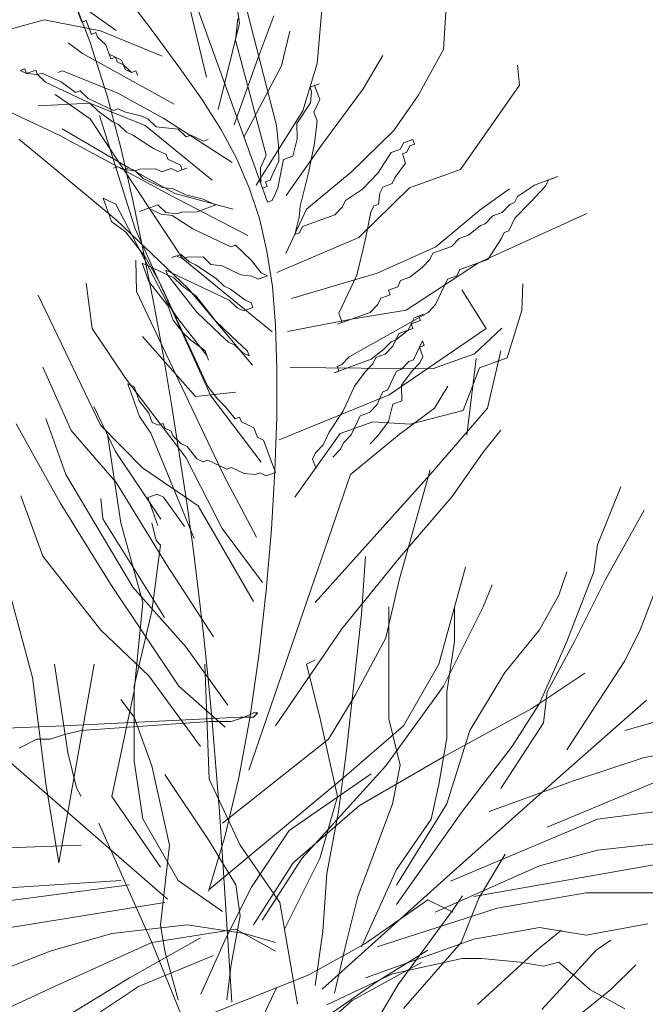
# Model space of a CAD drawing. Units: millimetres. Extents: x 595116 to 630915, y 909473 to 920225.
# Tile 61 of 134: x 629600.769 to 629604.389, y 919295.882 to 919301.582. Entities that reach past the tile are written whole.
import ezdxf

# ---------------------------------------------------------------- set-up
doc = ezdxf.new("R2010")
doc.units = ezdxf.units.MM
doc.layers.add('Dimension', color=3, linetype='Continuous', lineweight=18)
doc.layers.add('L-PLNT', color=85, linetype='Continuous', lineweight=13)
doc.styles.get("Standard").update_dxf_attribs({"font": 'arial.ttf'})
doc.dimstyles.new('ISO-25', dxfattribs={"dimtxt": 9, "dimasz": 6, "dimexe": 1.25, "dimexo": 0.625, "dimtad": 1, "dimlunit": 4, "dimtxsty": 'Standard', "dimcen": 2.5, "dimadec": 0, "dimazin": 0, "dimtfac": 1, "dimtmove": 0, "dimatfit": 3, "dimfxl": 1, "dimarcsym": 0})

# ---------------------------------------------------------------- blocks, each defined once
blk = doc.blocks.new('A$C4FB75ABC')
for p, q in [((2.7169, 3.7399), (2.6018, 4.2172)), ((2.8029, 3.5683), (2.5783, 4.1926)), ((2.7679, 3.8231), (2.7507, 3.9385)), ((2.7636, 3.9026), (2.8247, 3.6653)), ((2.5777, 3.8114), (2.4796, 3.8815)), ((2.5372, 3.7949), (2.5035, 3.8821)), ((2.5794, 3.8826), (2.6314, 3.8136)), ((2.8876, 3.7608), (2.897, 3.8696)), ((2.5166, 3.8462), (2.5244, 3.8247)), ((2.4664, 3.8281), (2.3706, 3.8017)), ((2.5536, 3.8109), (2.4664, 3.8281)), ((2.5244, 3.8247), (2.5315, 3.8272)), ((2.5315, 3.8272), (2.5393, 3.8057)), ((2.7613, 3.7965), (2.7653, 3.8303)), ((2.7957, 3.7683), (2.8207, 3.834)), ((3.0823, 3.7823), (3.0858, 3.8403)), ((2.6314, 3.8136), (2.6743, 3.7558)), ((2.7349, 3.6897), (2.7679, 3.8231)), ((2.5393, 3.8057), (2.5464, 3.8083)), ((2.5464, 3.8083), (2.549, 3.8011)), ((2.549, 3.8011), (2.5614, 3.7893)), ((2.6486, 3.7721), (2.5536, 3.8109)), ((2.8089, 3.6191), (2.7613, 3.7965)), ((2.8322, 3.7571), (2.8454, 3.8105)), ((2.5255, 3.7764), (2.5034, 3.7928)), ((2.5638, 3.7106), (2.5372, 3.7949)), ((2.5614, 3.7893), (2.5665, 3.775)), ((3.043, 3.7114), (3.0823, 3.7823)), ((2.6672, 3.6978), (2.5255, 3.7764)), ((2.5665, 3.775), (2.5763, 3.7704)), ((2.5691, 3.7678), (2.5665, 3.775)), ((2.5763, 3.7704), (2.5691, 3.7678)), ((2.5763, 3.7704), (2.5789, 3.7632)), ((2.586, 3.7658), (2.5763, 3.7704)), ((2.7596, 3.6662), (2.7957, 3.7683)), ((2.9584, 3.7215), (2.9885, 3.7729)), ((2.4369, 3.7526), (2.4297, 3.7501)), ((2.4394, 3.7455), (2.4369, 3.7526)), ((2.5789, 3.7632), (2.5886, 3.7586)), ((2.5886, 3.7586), (2.586, 3.7658)), ((2.5886, 3.7586), (2.5912, 3.7515)), ((2.601, 3.7469), (2.5886, 3.7586)), ((2.5912, 3.7515), (2.601, 3.7469)), ((2.6743, 3.7558), (2.7096, 3.7056)), ((2.7745, 3.6472), (2.8322, 3.7571)), ((2.8652, 3.6879), (2.8876, 3.7608)), ((3.1994, 3.7272), (3.1962, 3.7584)), ((2.4297, 3.7501), (2.4394, 3.7455)), ((2.4538, 3.7506), (2.4394, 3.7455)), ((2.4394, 3.7455), (2.4564, 3.7435)), ((2.4564, 3.7435), (2.4538, 3.7506)), ((2.4635, 3.746), (2.4564, 3.7435)), ((2.4564, 3.7435), (2.4687, 3.7317)), ((2.4733, 3.7414), (2.4635, 3.746)), ((2.4928, 3.7323), (2.4733, 3.7414)), ((2.4948, 3.7492), (2.4876, 3.7466)), ((2.58, 3.715), (2.4948, 3.7492)), ((2.601, 3.7469), (2.6081, 3.7494)), ((2.6081, 3.7494), (2.601, 3.7469)), ((2.6081, 3.7494), (2.6107, 3.7423)), ((2.6107, 3.7423), (2.6081, 3.7494)), ((2.4687, 3.7317), (2.4785, 3.7271)), ((2.4785, 3.7271), (2.498, 3.7179)), ((2.5149, 3.7159), (2.4928, 3.7323)), ((2.8907, 3.7295), (2.8764, 3.7244)), ((2.8764, 3.7244), (2.8789, 3.7172)), ((2.8835, 3.727), (2.8907, 3.7295)), ((2.8913, 3.7054), (2.8835, 3.727)), ((2.893, 3.6331), (2.9584, 3.7215)), ((3.1085, 3.5972), (3.1994, 3.7272)), ((2.5376, 3.6754), (2.4836, 3.7127)), ((2.498, 3.7179), (2.5272, 3.7041)), ((2.5221, 3.7185), (2.5149, 3.7159)), ((2.5344, 3.7067), (2.5221, 3.7185)), ((2.5441, 3.7021), (2.5344, 3.7067)), ((2.5853, 3.6284), (2.5638, 3.7106)), ((2.6509, 3.6757), (2.58, 3.715)), ((2.7096, 3.7056), (2.7388, 3.6597)), ((2.8789, 3.7172), (2.8769, 3.7003)), ((2.8821, 3.6859), (2.8913, 3.7054)), ((3.0058, 3.6575), (3.043, 3.7114)), ((2.537, 3.6995), (2.4575, 3.6952)), ((2.5272, 3.7041), (2.537, 3.6995)), ((2.537, 3.6995), (2.5493, 3.6877)), ((2.6222, 3.6653), (2.537, 3.6995)), ((2.5637, 3.6929), (2.5441, 3.7021)), ((2.5734, 3.6883), (2.5637, 3.6929)), ((2.5806, 3.6909), (2.5734, 3.6883)), ((2.5903, 3.6863), (2.5806, 3.6909)), ((2.8769, 3.7003), (2.856, 3.6684)), ((2.4899, 3.6502), (2.4119, 3.6869)), ((2.6801, 3.4593), (2.5376, 3.6754)), ((2.5493, 3.6877), (2.5714, 3.6714)), ((2.6067, 3.5058), (2.5519, 3.6806)), ((2.617, 3.6797), (2.5903, 3.6863)), ((2.6268, 3.6751), (2.617, 3.6797)), ((2.6391, 3.6633), (2.6268, 3.6751)), ((2.7562, 3.6082), (2.6509, 3.6757)), ((2.7932, 3.5729), (2.8652, 3.6879)), ((2.8873, 3.6716), (2.8821, 3.6859)), ((2.5972, 3.5996), (2.4945, 3.6599)), ((2.5714, 3.6714), (2.5812, 3.6668)), ((2.5812, 3.6668), (2.5935, 3.655)), ((2.7255, 3.5809), (2.6222, 3.6653)), ((2.673, 3.6593), (2.6391, 3.6633)), ((2.7388, 3.6597), (2.763, 3.6147)), ((2.8247, 3.6653), (2.8279, 3.634)), ((2.856, 3.6684), (2.8566, 3.6443)), ((2.8833, 3.6377), (2.8873, 3.6716)), ((2.5803, 3.6016), (2.4899, 3.6502)), ((2.5935, 3.655), (2.6032, 3.6504)), ((2.6032, 3.6504), (2.6351, 3.6295)), ((2.6853, 3.6475), (2.673, 3.6593)), ((2.6925, 3.6501), (2.6853, 3.6475)), ((2.7022, 3.6455), (2.6925, 3.6501)), ((2.712, 3.6409), (2.7022, 3.6455)), ((2.9398, 3.5932), (3.0058, 3.6575)), ((2.4618, 3.6157), (2.4274, 3.6439)), ((2.6351, 3.6295), (2.6448, 3.6249)), ((2.7192, 3.6435), (2.712, 3.6409)), ((2.8279, 3.634), (2.8285, 3.6099)), ((2.8394, 3.5571), (2.893, 3.6331)), ((2.8566, 3.6443), (2.85, 3.6176)), ((2.8746, 3.5941), (2.8833, 3.6377)), ((3.0207, 3.6385), (3.0161, 3.6288)), ((3.035, 3.6437), (3.0207, 3.6385)), ((3.0258, 3.6242), (3.0304, 3.6339)), ((3.0304, 3.6339), (3.0376, 3.6365)), ((3.0376, 3.6365), (3.035, 3.6437)), ((2.5774, 3.5196), (2.4618, 3.6157)), ((2.6037, 3.5475), (2.5853, 3.6284)), ((2.6448, 3.6249), (2.6546, 3.6203)), ((2.6546, 3.6203), (2.6572, 3.6131)), ((2.763, 3.6147), (2.7827, 3.5691)), ((2.7998, 3.5996), (2.8089, 3.6191)), ((2.85, 3.6176), (2.8356, 3.6125)), ((3.0017, 3.6236), (2.9808, 3.5918)), ((3.0161, 3.6288), (3.0017, 3.6236)), ((3.0187, 3.6216), (3.0258, 3.6242)), ((3.0238, 3.6072), (3.0187, 3.6216)), ((2.5803, 3.6016), (2.5731, 3.5991)), ((2.5731, 3.5991), (2.5803, 3.6016)), ((2.5901, 3.597), (2.5803, 3.6016)), ((2.5803, 3.6016), (2.5901, 3.597)), ((2.6609, 3.5577), (2.5803, 3.6016)), ((2.5972, 3.5996), (2.5901, 3.597)), ((2.607, 3.595), (2.5972, 3.5996)), ((2.6681, 3.5603), (2.5972, 3.5996)), ((2.6572, 3.6131), (2.6669, 3.6085)), ((2.6669, 3.6085), (2.6767, 3.6039)), ((2.6864, 3.5993), (2.6721, 3.5942)), ((2.6767, 3.6039), (2.6793, 3.5967)), ((2.6793, 3.5967), (2.6864, 3.5993)), ((2.8003, 3.5755), (2.7998, 3.5996)), ((2.8285, 3.6099), (2.8193, 3.5904)), ((2.8356, 3.6125), (2.827, 3.5688)), ((3.0075, 3.5852), (3.0238, 3.6072)), ((2.5901, 3.597), (2.607, 3.595)), ((2.6142, 3.5976), (2.607, 3.595)), ((2.607, 3.595), (2.6193, 3.5833)), ((2.6383, 3.5982), (2.6142, 3.5976)), ((2.648, 3.5936), (2.6383, 3.5982)), ((2.6623, 3.5987), (2.648, 3.5936)), ((2.6721, 3.5942), (2.6623, 3.5987)), ((2.8193, 3.5904), (2.8147, 3.5806)), ((2.868, 3.5674), (2.8746, 3.5941)), ((2.8712, 3.5361), (2.9398, 3.5932)), ((2.9808, 3.5918), (2.969, 3.5794)), ((3.0029, 3.5754), (3.0075, 3.5852)), ((3.0296, 3.5688), (3.1085, 3.5972)), ((3.2582, 3.5862), (3.2224, 3.5733)), ((3.2439, 3.5811), (3.2582, 3.5862)), ((2.6193, 3.5833), (2.6486, 3.5695)), ((2.6486, 3.5695), (2.6655, 3.5675)), ((2.7827, 3.5691), (2.7983, 3.5216)), ((2.8107, 3.5468), (2.8003, 3.5755)), ((2.8101, 3.5709), (2.8029, 3.5683)), ((2.8147, 3.5806), (2.8075, 3.578)), ((2.8075, 3.578), (2.8101, 3.5709)), ((2.827, 3.5688), (2.8224, 3.5591)), ((2.9518, 3.4922), (3.0296, 3.5688)), ((2.969, 3.5794), (2.9573, 3.5671)), ((2.984, 3.5605), (2.9885, 3.5702)), ((2.9885, 3.5702), (3.0029, 3.5754)), ((3.2224, 3.5733), (3.1962, 3.5558)), ((3.2158, 3.5466), (3.2393, 3.5713)), ((3.2393, 3.5713), (3.2439, 3.5811)), ((2.7805, 3.4954), (2.6609, 3.5577)), ((2.6655, 3.5675), (2.685, 3.5583)), ((2.7579, 3.5359), (2.6681, 3.5603)), ((2.685, 3.5583), (2.7117, 3.5517)), ((2.8224, 3.5591), (2.8178, 3.5493)), ((2.8614, 3.5407), (2.868, 3.5674)), ((2.9573, 3.5671), (2.9312, 3.5496)), ((2.9819, 3.5435), (2.984, 3.5605)), ((3.1389, 3.5352), (3.1839, 3.5676)), ((3.1962, 3.5558), (3.1917, 3.5461)), ((2.5671, 3.5483), (2.5573, 3.5529)), ((2.5573, 3.5529), (2.5703, 3.517)), ((2.5769, 3.5437), (2.5671, 3.5483)), ((2.6552, 3.3935), (2.5769, 3.5437)), ((2.6204, 3.467), (2.6037, 3.5475)), ((2.642, 3.5428), (2.6133, 3.5325)), ((2.6543, 3.531), (2.642, 3.5428)), ((2.7312, 3.5425), (2.7025, 3.5321)), ((2.7117, 3.5517), (2.7214, 3.5471)), ((2.7214, 3.5471), (2.7312, 3.5425)), ((2.8178, 3.5493), (2.8107, 3.5468)), ((2.8594, 3.5238), (2.8614, 3.5407)), ((2.9266, 3.5398), (2.9148, 3.5275)), ((2.9312, 3.5496), (2.9266, 3.5398)), ((2.9702, 3.5312), (2.9748, 3.541)), ((2.9748, 3.541), (2.9819, 3.5435)), ((3.1845, 3.5435), (3.1727, 3.5311)), ((3.1917, 3.5461), (3.1845, 3.5435)), ((3.1922, 3.522), (3.2158, 3.5466)), ((2.6133, 3.5325), (2.6276, 3.5376)), ((2.6276, 3.5376), (2.6471, 3.5284)), ((2.6471, 3.5284), (2.6641, 3.5264)), ((2.6712, 3.529), (2.6543, 3.531)), ((2.6641, 3.5264), (2.6959, 3.5055)), ((2.6784, 3.5316), (2.6712, 3.529)), ((2.7025, 3.5321), (2.6784, 3.5316)), ((2.8391, 3.4678), (2.8712, 3.5361)), ((2.8528, 3.4971), (2.8594, 3.5238)), ((2.9148, 3.5275), (2.8646, 3.5094)), ((2.9616, 3.4876), (2.9702, 3.5312)), ((3.0703, 3.4781), (3.1389, 3.5352)), ((3.136, 3.4531), (3.303, 3.5294)), ((3.1584, 3.526), (3.1466, 3.5136)), ((3.1727, 3.5311), (3.1584, 3.526)), ((2.5703, 3.517), (2.5924, 3.5006)), ((2.6885, 3.4136), (2.5774, 3.5196)), ((2.7983, 3.5216), (2.81, 3.4712)), ((2.8646, 3.5094), (2.86, 3.4997)), ((3.1394, 3.5111), (3.1205, 3.4961)), ((3.1466, 3.5136), (3.1394, 3.5111)), ((3.1831, 3.5024), (3.1922, 3.522)), ((2.5924, 3.5006), (2.6222, 3.4627)), ((2.7237, 3.248), (2.6067, 3.5058)), ((2.6959, 3.5055), (2.7154, 3.4963)), ((2.7154, 3.4963), (2.7252, 3.4917)), ((2.86, 3.4997), (2.8528, 3.4971)), ((3.1205, 3.4961), (3.1062, 3.491)), ((3.1713, 3.4901), (3.1759, 3.4999)), ((3.1759, 3.4999), (3.1831, 3.5024)), ((2.7252, 3.4917), (2.7544, 3.4779)), ((2.7544, 3.4779), (2.7616, 3.4805)), ((2.7616, 3.4805), (2.774, 3.4687)), ((2.8253, 3.4385), (2.9518, 3.4922)), ((2.9484, 3.4342), (2.9616, 3.4876)), ((2.9797, 3.4374), (3.0703, 3.4781)), ((3.0944, 3.4786), (3.0657, 3.4683)), ((3.1062, 3.491), (3.0944, 3.4786)), ((3.1503, 3.4583), (3.1713, 3.4901)), ((2.636, 3.3873), (2.6204, 3.467)), ((2.6222, 3.4627), (2.6449, 3.4222)), ((2.6632, 3.4613), (2.6776, 3.4664)), ((2.6704, 3.4639), (2.6632, 3.4613)), ((2.6801, 3.4593), (2.6704, 3.4639)), ((2.6776, 3.4664), (2.6899, 3.4547)), ((2.7114, 3.4624), (2.6873, 3.4618)), ((2.7237, 3.4506), (2.7114, 3.4624)), ((2.774, 3.4687), (2.7863, 3.4569)), ((2.81, 3.4712), (2.8183, 3.4166)), ((3.0657, 3.4683), (3.0611, 3.4586)), ((2.609, 3.4093), (2.6078, 3.4576)), ((2.6566, 3.4346), (2.6176, 3.453)), ((2.6176, 3.453), (2.6279, 3.4243)), ((2.6873, 3.4618), (2.6801, 3.4593)), ((2.8178, 3.3467), (2.6801, 3.4593)), ((2.6899, 3.4547), (2.6996, 3.4501)), ((2.6996, 3.4501), (2.7315, 3.4291)), ((2.7407, 3.4486), (2.7237, 3.4506)), ((2.7699, 3.4348), (2.7407, 3.4486)), ((2.7863, 3.4569), (2.8012, 3.438)), ((3.0244, 3.3805), (3.136, 3.4531)), ((3.0611, 3.4586), (3.0494, 3.4462)), ((3.1073, 3.4428), (3.1503, 3.4583)), ((2.6638, 3.4372), (2.654, 3.4418)), ((2.654, 3.4418), (2.6566, 3.4346)), ((2.6566, 3.4346), (2.6664, 3.43)), ((2.6865, 3.3967), (2.6566, 3.4346)), ((2.693, 3.4234), (2.6638, 3.4372)), ((2.7869, 3.4328), (2.7699, 3.4348)), ((2.7966, 3.4282), (2.7869, 3.4328)), ((2.811, 3.4334), (2.7966, 3.4282)), ((2.8012, 3.438), (2.811, 3.4334)), ((2.848, 3.3981), (2.9797, 3.4374)), ((2.9392, 3.4147), (2.9484, 3.4342)), ((3.0494, 3.4462), (3.0304, 3.4313)), ((3.0884, 3.4279), (3.1027, 3.433)), ((3.1027, 3.433), (3.1073, 3.4428)), ((2.5404, 3.3522), (2.5315, 3.422)), ((2.6279, 3.4243), (2.6578, 3.3864)), ((2.6449, 3.4222), (2.7186, 3.2624)), ((2.6664, 3.43), (2.6787, 3.4182)), ((2.6787, 3.4182), (2.7008, 3.4019)), ((2.7028, 3.4188), (2.693, 3.4234)), ((2.7223, 3.4096), (2.7028, 3.4188)), ((2.7315, 3.4291), (2.7438, 3.4173)), ((2.7438, 3.4173), (2.7536, 3.4127)), ((3.0161, 3.4262), (3.0115, 3.4164)), ((3.0304, 3.4313), (3.0161, 3.4262)), ((3.07, 3.3888), (3.0884, 3.4279)), ((3.2028, 3.3799), (3.2043, 3.4209)), ((2.5536, 3.203), (2.4572, 3.4034)), ((2.6446, 3.333), (2.609, 3.4093)), ((2.7877, 3.2953), (2.6885, 3.4136)), ((2.7008, 3.4019), (2.7306, 3.364)), ((2.7516, 3.3958), (2.7223, 3.4096)), ((2.7536, 3.4127), (2.7757, 3.3964)), ((2.8183, 3.4166), (2.8233, 3.3565)), ((2.9254, 3.3854), (2.9392, 3.4147)), ((2.9997, 3.4041), (2.9854, 3.3989)), ((3.0115, 3.4164), (2.9972, 3.4112)), ((2.9972, 3.4112), (2.9997, 3.4041)), ((3.1481, 3.3521), (3.1105, 3.4115)), ((2.6503, 3.3086), (2.636, 3.3873)), ((2.6727, 3.3674), (2.6552, 3.3935)), ((2.6578, 3.3864), (2.6655, 3.3648)), ((2.7014, 3.3777), (2.6865, 3.3967)), ((2.7639, 3.384), (2.7516, 3.3958)), ((2.7757, 3.3964), (2.7854, 3.3918)), ((2.7854, 3.3918), (2.788, 3.3846)), ((2.9808, 3.3891), (2.969, 3.3768)), ((2.9854, 3.3989), (2.9808, 3.3891)), ((3.0583, 3.3765), (3.07, 3.3888)), ((2.7384, 3.3424), (2.7014, 3.3777)), ((2.7737, 3.3794), (2.7639, 3.384)), ((2.788, 3.3846), (2.7737, 3.3794)), ((2.969, 3.3768), (2.9188, 3.3587)), ((2.9208, 3.3757), (2.9254, 3.3854)), ((2.926, 3.3613), (2.9208, 3.3757)), ((2.9369, 3.3085), (3.0583, 3.3765)), ((2.9403, 3.3665), (3.0244, 3.3805)), ((3.0511, 3.3739), (3.0367, 3.3687)), ((3.0439, 3.3713), (3.0511, 3.3739)), ((3.0465, 3.3642), (3.0439, 3.3713)), ((3.1805, 3.307), (3.2028, 3.3799)), ((2.6655, 3.3648), (2.6804, 3.3459)), ((2.7174, 3.3106), (2.6727, 3.3674)), ((2.7306, 3.364), (2.743, 3.3522)), ((2.8233, 3.3565), (2.8254, 3.2898)), ((2.8419, 3.3473), (2.9403, 3.3665)), ((2.9188, 3.3587), (2.926, 3.3613)), ((3.0322, 3.359), (3.0276, 3.3492)), ((3.0367, 3.3687), (3.0322, 3.359)), ((3.0322, 3.359), (3.0465, 3.3642)), ((3.0347, 3.3518), (3.0322, 3.359)), ((2.5929, 3.2739), (2.5404, 3.3522)), ((2.6804, 3.3459), (2.6928, 3.3341)), ((2.7507, 3.3307), (2.7384, 3.3424)), ((2.743, 3.3522), (2.7553, 3.3404)), ((2.9986, 3.2497), (3.1481, 3.3521)), ((3.0276, 3.3492), (3.0086, 3.3343)), ((3.0086, 3.3343), (3.0132, 3.3441)), ((3.0132, 3.3441), (3.0347, 3.3518)), ((3.1297, 3.313), (3.1722, 3.3526)), ((2.6997, 3.2474), (2.6179, 3.3396)), ((2.7435, 3.1255), (2.6446, 3.333)), ((2.6928, 3.3341), (2.7149, 3.3178)), ((2.7605, 3.3261), (2.7507, 3.3307)), ((2.7553, 3.3404), (2.78, 3.3169)), ((2.7728, 3.3143), (2.7605, 3.3261)), ((3.0015, 3.3317), (2.9897, 3.3194)), ((3.0086, 3.3343), (3.0015, 3.3317)), ((3.004, 3.3246), (3.0086, 3.3343)), ((3.0497, 3.3329), (3.0451, 3.3231)), ((3.0451, 3.3231), (3.0522, 3.3257)), ((3.0522, 3.3257), (3.0497, 3.3329)), ((2.7149, 3.3178), (2.72, 3.3034)), ((2.72, 3.3034), (2.7174, 3.3106)), ((2.7826, 3.3097), (2.7728, 3.3143)), ((2.78, 3.3169), (2.7826, 3.3097)), ((2.9897, 3.3194), (2.9708, 3.3045)), ((2.9779, 3.3071), (2.9923, 3.3122)), ((2.9923, 3.3122), (3.004, 3.3246)), ((3.0359, 3.3036), (3.0405, 3.3134)), ((3.0405, 3.3134), (3.0451, 3.3231)), ((3.0451, 3.3231), (3.0502, 3.3088)), ((3.0651, 3.2898), (3.1297, 3.313)), ((3.1501, 3.2292), (3.1706, 3.3178)), ((2.6635, 3.2315), (2.6503, 3.3086)), ((2.9708, 3.3045), (2.9134, 3.2838)), ((2.918, 3.2936), (2.9251, 3.2962)), ((2.9251, 3.2962), (2.9369, 3.3085)), ((2.9616, 3.285), (2.9733, 3.2973)), ((2.9733, 3.2973), (2.9779, 3.3071)), ((3.0169, 3.2887), (3.0287, 3.301)), ((3.0287, 3.301), (3.0359, 3.3036)), ((3.0456, 3.299), (3.0339, 3.2867)), ((3.0502, 3.3088), (3.0456, 3.299)), ((3.1303, 3.2889), (3.1323, 3.3059)), ((3.1374, 3.2915), (3.1805, 3.307)), ((2.508, 3.1947), (2.4647, 3.2926)), ((2.8254, 3.2898), (2.825, 3.2153)), ((2.8457, 3.2919), (3.0651, 3.2898)), ((2.9134, 3.2838), (2.9206, 3.2864)), ((2.9206, 3.2864), (2.918, 3.2936)), ((2.9452, 3.2629), (2.9616, 3.285)), ((3.0052, 3.2763), (3.0098, 3.2861)), ((3.0098, 3.2861), (3.0169, 3.2887)), ((3.0339, 3.2867), (3.0175, 3.2646)), ((3.1125, 3.2258), (3.1374, 3.2915)), ((3.1182, 3.1873), (3.1303, 3.2889)), ((2.685, 3.153), (2.5929, 3.2739)), ((2.6053, 3.2621), (2.5955, 3.2667)), ((2.5955, 3.2667), (2.6136, 3.2165)), ((2.996, 3.2568), (3.0052, 3.2763)), ((2.613, 3.2406), (2.6053, 3.2621)), ((2.7622, 3.2537), (2.6997, 3.2474)), ((2.7186, 3.2624), (2.7335, 3.2434)), ((2.829, 3.1805), (2.9986, 3.2497)), ((2.936, 3.2434), (2.9452, 3.2629)), ((2.9842, 3.2445), (2.9888, 3.2542)), ((2.9888, 3.2542), (2.996, 3.2568)), ((3.0175, 3.2646), (3.0181, 3.2405)), ((3.0684, 3.2292), (3.0888, 3.2633)), ((2.6279, 3.2216), (2.613, 3.2406)), ((2.8009, 3.1461), (2.7237, 3.248)), ((2.7335, 3.2434), (2.7458, 3.2316)), ((2.9269, 3.2238), (2.936, 3.2434)), ((2.9679, 3.2224), (2.9797, 3.2347)), ((2.9797, 3.2347), (2.9842, 3.2445)), ((3.0038, 3.2353), (2.9972, 3.2086)), ((3.0181, 3.2405), (3.0038, 3.2353)), ((2.5763, 3.1625), (2.5433, 3.2317)), ((2.6331, 3.2073), (2.6279, 3.2216)), ((2.6754, 3.1561), (2.6635, 3.2315)), ((2.7458, 3.2316), (2.7608, 3.2127)), ((2.9059, 3.192), (2.9269, 3.2238)), ((2.9535, 3.2172), (2.9679, 3.2224)), ((3.0139, 3.1884), (3.0684, 3.2292)), ((3.031, 3.2046), (3.1125, 3.2258)), ((3.0616, 3.1271), (3.1501, 3.2292)), ((2.4914, 3.0833), (2.4234, 3.2048)), ((2.5, 3.127), (2.469, 3.2131)), ((2.6136, 3.2165), (2.6311, 3.1904)), ((2.6428, 3.2027), (2.6331, 3.2073)), ((2.65, 3.2053), (2.6428, 3.2027)), ((2.6526, 3.1981), (2.65, 3.2053)), ((2.7608, 3.2127), (2.7679, 3.2153)), ((2.7679, 3.2153), (2.7705, 3.2081)), ((2.7705, 3.2081), (2.7803, 3.2035)), ((2.825, 3.2153), (2.8223, 3.1323)), ((2.9229, 3.19), (2.9731, 3.208)), ((2.9398, 3.188), (2.949, 3.2075)), ((2.949, 3.2075), (2.9535, 3.2172)), ((2.9731, 3.208), (3.031, 3.2046)), ((2.9972, 3.2086), (2.9808, 3.1865)), ((2.5774, 3.1143), (2.508, 3.1947)), ((2.6179, 3.137), (2.5536, 3.203)), ((2.6311, 3.1904), (2.6976, 3.0279)), ((2.6624, 3.1935), (2.6526, 3.1981)), ((2.6649, 3.1863), (2.6624, 3.1935)), ((2.7803, 3.2035), (2.79, 3.1989)), ((2.79, 3.1989), (2.7952, 3.1846)), ((2.8529, 3.0918), (2.9229, 3.19)), ((2.8967, 3.1725), (2.9059, 3.192)), ((3.1433, 3.1611), (3.1706, 3.1952)), ((2.5847, 3.0522), (2.5642, 3.1884)), ((2.6773, 3.1746), (2.6649, 3.1863)), ((2.687, 3.17), (2.6773, 3.1746)), ((2.7952, 3.1846), (2.8049, 3.18)), ((2.8049, 3.18), (2.823, 3.1297)), ((2.9234, 3.1659), (2.928, 3.1756)), ((2.928, 3.1756), (2.9398, 3.188)), ((2.9389, 3.1271), (3.0139, 3.1884)), ((2.9808, 3.1865), (2.969, 3.1742)), ((2.6463, 3.058), (2.5763, 3.1625)), ((2.7019, 3.151), (2.687, 3.17)), ((2.8804, 3.1504), (2.885, 3.1601)), ((2.885, 3.1601), (2.8967, 3.1725)), ((2.9117, 3.1535), (2.9234, 3.1659)), ((3.0956, 3.093), (3.1433, 3.1611)), ((2.6863, 3.0831), (2.6754, 3.1561)), ((2.7407, 3.0434), (2.685, 3.153)), ((2.7117, 3.1464), (2.7019, 3.151)), ((2.7189, 3.149), (2.7117, 3.1464)), ((2.7286, 3.1444), (2.7189, 3.149)), ((2.7481, 3.1352), (2.7286, 3.1444)), ((2.8856, 3.136), (2.8804, 3.1504)), ((2.7037, 3.0787), (2.6179, 3.137)), ((2.7553, 3.1378), (2.7481, 3.1352)), ((2.7651, 3.1332), (2.7553, 3.1378)), ((2.7748, 3.1286), (2.7651, 3.1332)), ((2.7917, 3.1266), (2.7748, 3.1286)), ((2.7989, 3.1292), (2.7917, 3.1266)), ((2.8087, 3.1246), (2.7989, 3.1292)), ((2.823, 3.1297), (2.8087, 3.1246)), ((2.8223, 3.1323), (2.817, 3.0425)), ((3.0139, 2.9637), (3.0616, 3.1339)), ((2.603, 2.9533), (2.5, 3.127)), ((2.6552, 2.9883), (2.5774, 3.1143)), ((2.794, 3.0302), (2.7435, 3.1255)), ((2.7823, 2.6709), (2.9389, 3.1271)), ((2.8844, 2.9296), (3.0616, 3.1271)), ((3.3198, 3.0184), (3.3556, 3.1078)), ((2.4644, 3.0007), (2.4308, 3.094)), ((2.5691, 2.9573), (2.4914, 3.0833)), ((2.5571, 3.0584), (2.5539, 3.0896)), ((2.6406, 3.0965), (2.6262, 3.0913)), ((2.6262, 3.0913), (2.6417, 3.0483)), ((2.6503, 3.0919), (2.6406, 3.0965)), ((2.6827, 3.0468), (2.6503, 3.0919)), ((2.696, 3.0126), (2.6863, 3.0831)), ((3.0139, 2.9977), (3.0956, 3.093)), ((2.7892, 2.9311), (2.7037, 3.0787)), ((3.3317, 2.9647), (3.3914, 3.072)), ((2.6523, 2.9062), (2.5571, 3.0584)), ((2.6187, 2.9296), (2.5847, 3.0522)), ((2.6392, 3.0249), (2.6324, 3.0522)), ((2.8029, 2.9604), (2.7407, 3.0434)), ((2.817, 3.0425), (2.809, 2.948)), ((2.646, 3.0181), (2.6392, 3.0249)), ((2.6324, 2.916), (2.646, 3.0181)), ((2.7046, 2.9452), (2.696, 3.0126)), ((3.3138, 2.9766), (3.3198, 3.0184)), ((2.5539, 2.887), (2.4644, 3.0007)), ((2.9253, 2.8888), (3.0139, 2.9977)), ((2.9559, 2.911), (2.9619, 3.0005)), ((2.4007, 2.9909), (2.4484, 2.8139)), ((2.7278, 2.8766), (2.6552, 2.9883)), ((3.0752, 2.8343), (3.1161, 2.9841)), ((3.2601, 2.9408), (3.2721, 2.9766)), ((3.2721, 2.8693), (3.3138, 2.9766)), ((2.9935, 2.8751), (3.0139, 2.9637)), ((3.284, 2.8693), (3.3317, 2.9647)), ((3.3854, 2.8872), (3.4152, 2.9647)), ((2.6741, 2.8006), (2.5691, 2.9573)), ((2.6847, 2.8611), (2.603, 2.9533)), ((2.809, 2.948), (2.7981, 2.8512)), ((3.1433, 2.9228), (3.157, 2.9569)), ((2.7122, 2.8807), (2.7046, 2.9452)), ((3.2303, 2.8872), (3.2601, 2.9408)), ((2.6051, 2.7934), (2.6187, 2.9296)), ((2.6051, 2.8002), (2.6324, 2.916)), ((2.9977, 2.8216), (2.9977, 2.923)), ((3.082, 2.8002), (3.1433, 2.9228)), ((3.0991, 2.8693), (3.0991, 2.923)), ((2.944, 2.8037), (2.9559, 2.911)), ((2.6279, 2.8164), (2.5539, 2.887)), ((2.8231, 2.739), (2.9253, 2.8888)), ((3.1766, 2.8216), (3.2303, 2.8872)), ((3.3615, 2.8395), (3.3854, 2.8872)), ((2.7189, 2.8171), (2.7122, 2.8807)), ((2.9458, 2.7866), (2.9935, 2.8751)), ((2.7496, 2.771), (2.6847, 2.8611)), ((3.0872, 2.7918), (3.0991, 2.8693)), ((3.2303, 2.7739), (3.2721, 2.8693)), ((3.2422, 2.7918), (3.284, 2.8693)), ((2.7981, 2.8512), (2.784, 2.7542)), ((2.8708, 2.8343), (2.8844, 2.8411)), ((2.4825, 2.8343), (2.5029, 2.6981)), ((2.4893, 2.5279), (2.5438, 2.8343)), ((2.7209, 2.6572), (2.7141, 2.8343)), ((2.8913, 2.7526), (2.8708, 2.8343)), ((3.0207, 2.739), (3.0752, 2.8343)), ((3.2721, 2.7024), (3.3615, 2.8395)), ((2.4484, 2.8139), (2.4689, 2.6504)), ((2.7077, 2.7073), (2.6279, 2.8164)), ((2.7251, 2.7519), (2.7189, 2.8171)), ((2.9977, 2.7501), (2.9977, 2.8216)), ((3.1229, 2.7322), (3.1766, 2.8216)), ((3.2183, 2.7662), (3.3, 2.8207)), ((2.6051, 2.6845), (2.6051, 2.8002)), ((2.7456, 2.7371), (2.6741, 2.8006)), ((2.9321, 2.6964), (2.944, 2.8037)), ((2.9935, 2.6777), (3.082, 2.8002)), ((2.5711, 2.63), (2.6051, 2.7934)), ((2.6051, 2.7526), (2.5847, 2.7798)), ((2.9049, 2.7185), (2.9458, 2.7866)), ((3.0872, 2.7203), (3.0872, 2.7918)), ((3.2363, 2.7441), (3.2422, 2.7918)), ((3.2623, 2.6619), (3.3951, 2.779)), ((3.082, 2.6913), (3.2183, 2.7662)), ((3.1886, 2.7083), (3.2303, 2.7739)), ((3.3615, 2.7322), (3.5107, 2.7739)), ((2.4961, 2.739), (2.7686, 2.7526)), ((2.6324, 2.6777), (2.6051, 2.7526)), ((2.7309, 2.6826), (2.7251, 2.7519)), ((2.7754, 2.7526), (2.755, 2.7458)), ((2.784, 2.7542), (2.7664, 2.6591)), ((2.7686, 2.7526), (2.7891, 2.7526)), ((2.7891, 2.7594), (2.7754, 2.7526)), ((2.7891, 2.7526), (2.7959, 2.7594)), ((2.7959, 2.7594), (2.7891, 2.7594)), ((2.9185, 2.63), (2.8913, 2.7526)), ((3.0156, 2.6785), (2.9977, 2.7501)), ((2.3122, 2.7321), (2.4961, 2.739)), ((2.7209, 2.7458), (2.5234, 2.7321)), ((2.755, 2.7458), (2.7209, 2.7458)), ((2.9253, 2.6572), (3.0207, 2.739)), ((3.1707, 2.6428), (3.2363, 2.7441)), ((2.4552, 2.7185), (2.428, 2.7049)), ((2.4757, 2.7185), (2.4552, 2.7185)), ((2.4961, 2.7253), (2.4757, 2.7185)), ((2.5234, 2.7321), (2.4961, 2.7253)), ((2.7414, 2.5891), (2.9049, 2.7185)), ((3.0752, 2.6487), (3.0872, 2.7203)), ((3.0872, 2.6189), (3.1229, 2.7322)), ((3.111, 2.607), (3.1886, 2.7083)), ((2.6566, 2.472), (2.3943, 2.7002)), ((2.5029, 2.6981), (2.5166, 2.6436)), ((2.9201, 2.607), (2.9321, 2.6964)), ((2.9526, 2.6164), (3.082, 2.6913)), ((3.2422, 2.5831), (3.4987, 2.6904)), ((3.284, 2.6547), (3.3914, 2.6904)), ((3.3914, 2.6904), (3.4629, 2.7024)), ((2.6187, 2.596), (2.6051, 2.6845)), ((2.6596, 2.5551), (2.6324, 2.6777)), ((2.7367, 2.6065), (2.7309, 2.6826)), ((2.864, 2.5347), (2.9935, 2.6777)), ((3.0036, 2.6189), (3.0156, 2.6785)), ((2.6528, 2.664), (2.7209, 2.5619)), ((2.7664, 2.6591), (2.7451, 2.5683)), ((2.8442, 2.5778), (2.9704, 2.6651)), ((3.0976, 2.5149), (3.2623, 2.6619)), ((2.4689, 2.6504), (2.4893, 2.5279)), ((2.5166, 2.6436), (2.5234, 2.63)), ((2.7209, 2.487), (2.9253, 2.6572)), ((2.7686, 2.5551), (2.7209, 2.6572)), ((3.0633, 2.5951), (3.0752, 2.6487)), ((3.1528, 2.607), (3.284, 2.6547)), ((2.646, 2.5211), (2.5711, 2.63)), ((2.8913, 2.5347), (2.9185, 2.63)), ((2.8504, 2.5279), (2.9526, 2.6164)), ((2.95, 2.4758), (3.0036, 2.6189)), ((3.0096, 2.4937), (3.0872, 2.6189)), ((3.3198, 2.5951), (3.457, 2.6129)), ((2.7426, 2.5213), (2.7367, 2.6065)), ((2.9022, 2.5116), (2.9201, 2.607)), ((3.0096, 2.4639), (3.111, 2.607)), ((2.5506, 2.5891), (2.6324, 2.4053)), ((2.6732, 2.5006), (2.6187, 2.596)), ((3.0096, 2.5176), (3.0633, 2.5951)), ((3.0931, 2.4997), (3.3198, 2.5951)), ((2.7451, 2.5683), (2.72, 2.484)), ((2.786, 2.4905), (2.8442, 2.5778)), ((2.5234, 2.5551), (2.1282, 2.5415)), ((2.646, 2.4325), (2.6596, 2.5551)), ((2.7209, 2.5619), (2.7618, 2.4938)), ((2.8299, 2.4666), (2.7686, 2.5551)), ((3.3198, 2.5474), (3.4272, 2.5593)), ((3.1289, 2.4758), (3.5345, 2.5474)), ((3.1365, 2.4734), (3.1774, 2.5415)), ((3.2303, 2.5235), (3.3198, 2.5474)), ((2.7489, 2.4244), (2.7426, 2.5213)), ((2.7891, 2.4325), (2.8504, 2.5279)), ((2.8027, 2.4393), (2.864, 2.5347)), ((2.8368, 2.4257), (2.8913, 2.5347)), ((3.0693, 2.452), (3.2303, 2.5235)), ((2.895, 2.333), (3.0976, 2.5149)), ((2.8963, 2.4222), (2.9022, 2.5116)), ((2.9559, 2.3983), (3.0096, 2.5176)), ((2.5847, 2.5006), (2.1555, 2.4734)), ((2.5983, 2.4938), (2.1827, 2.4393)), ((2.7414, 2.453), (2.6732, 2.5006)), ((2.7471, 2.4129), (2.786, 2.4905)), ((2.7618, 2.4938), (2.7686, 2.4461)), ((2.9321, 2.4043), (2.95, 2.4758)), ((3.0962, 2.4544), (3.1115, 2.4773)), ((3.1647, 2.4579), (3.3019, 2.4818)), ((3.3019, 2.4818), (3.4152, 2.4818)), ((2.6528, 2.4666), (2.1895, 2.3917)), ((2.8572, 2.31), (2.8299, 2.4666)), ((2.9607, 2.4032), (3.0578, 2.4711)), ((3.0578, 2.4711), (3.0966, 2.4517)), ((3.1093, 2.4053), (3.1365, 2.4734)), ((2.7686, 2.4461), (2.755, 2.3712)), ((2.9798, 2.3983), (3.1647, 2.4579)), ((3.0123, 2.3401), (3.0962, 2.4544)), ((2.5711, 2.4189), (2.6869, 2.4325)), ((2.6528, 2.3917), (2.646, 2.4325)), ((2.6869, 2.4325), (2.7754, 2.4189)), ((3.3019, 2.4162), (3.3973, 2.4341)), ((2.4757, 2.3917), (2.5711, 2.4189)), ((2.6324, 2.4053), (2.7618, 2.4257)), ((2.7559, 2.3132), (2.7489, 2.4244)), ((2.7618, 2.4257), (2.8231, 2.3917)), ((2.7754, 2.4189), (2.8231, 2.4053)), ((2.8844, 2.3387), (2.8963, 2.4222)), ((3.1289, 2.4102), (3.2303, 2.4281)), ((3.2259, 2.3934), (3.264, 2.4239)), ((3.2303, 2.4281), (3.3019, 2.4162)), ((2.4825, 2.3372), (2.6324, 2.4053)), ((2.7073, 2.4121), (2.5983, 2.3508)), ((2.6324, 2.4053), (2.7073, 2.2214)), ((2.7083, 2.3255), (2.7471, 2.4129)), ((2.8733, 2.3546), (2.9607, 2.4032)), ((2.9142, 2.3268), (2.9321, 2.4043)), ((2.9619, 2.3506), (3.1289, 2.4102)), ((3.0207, 2.3031), (3.1093, 2.4053)), ((3.3174, 2.3934), (3.3403, 2.4087)), ((2.353, 2.344), (2.4757, 2.3917)), ((2.7277, 2.3849), (2.6119, 2.3372)), ((2.6732, 2.3168), (2.6528, 2.3917)), ((2.9801, 2.3449), (3.0578, 2.3935)), ((3.1344, 2.3096), (3.2259, 2.3934)), ((3.2335, 2.302), (3.3174, 2.3934)), ((2.755, 2.3712), (2.7482, 2.3168)), ((2.9413, 2.3158), (3.0481, 2.3741)), ((3.0036, 2.3566), (3.111, 2.3804)), ((3.111, 2.3804), (3.1408, 2.3804)), ((3.1408, 2.3804), (3.2005, 2.3745)), ((3.2005, 2.3745), (3.2363, 2.3685)), ((3.2363, 2.3685), (3.2601, 2.3745)), ((3.2601, 2.3745), (3.3079, 2.3327)), ((3.3403, 2.3324), (3.3784, 2.3706)), ((2.7277, 2.2964), (2.8733, 2.3546)), ((2.9022, 2.3089), (3.0036, 2.3566)), ((2.5983, 2.3508), (2.4757, 2.2759)), ((2.8539, 2.2576), (2.9801, 2.3449)), ((2.9666, 2.2638), (3.0123, 2.3401)), ((2.3054, 2.2555), (2.4825, 2.3372)), ((2.6119, 2.3372), (2.5302, 2.2827)), ((2.8248, 2.3352), (2.7471, 2.1703)), ((3.264, 2.2715), (3.3403, 2.3324)), ((3.3079, 2.3327), (3.3615, 2.3029)), ((2.8539, 2.2382), (2.9413, 2.3158))]:
    blk.add_line(p, q)
blk = doc.blocks.new('*D210')
at = {"layer": 'Defpoints', "color": 0, "transparency": 16777216}
for p in [(629586.2273, 919310.1229), (629593.9463, 919310.1229), (629586.2273, 919258.6624)]:
    blk.add_point(p, dxfattribs=at)
at = {"layer": 'Dimension', "color": 0, "lineweight": -2, "transparency": 16777216}
for p, q in [((629593.9463, 919310.1229), (629593.9463, 919449.6901)), ((629586.8523, 919310.1229), (629595.1963, 919310.1229)), ((629593.9463, 919264.6624), (629593.9463, 919304.1229)), ((629586.8523, 919258.6624), (629595.1963, 919258.6624))]:
    blk.add_line(p, q, dxfattribs=at)
at = {"layer": 'Dimension', "color": 0, "transparency": 16777216}
for points in [[(629592.9463, 919304.1229), (629594.9463, 919304.1229), (629593.9463, 919310.1229)], [(629592.9463, 919264.6624), (629594.9463, 919264.6624), (629593.9463, 919258.6624)]]:
    blk.add_solid(points, dxfattribs=at)
at = {"layer": 'Dimension', "color": 0, "transparency": 16777216, "insert": (629588.6617, 919382.9065), "char_height": 9, "attachment_point": 5, "rotation": 90}
blk.add_mtext('CANOPY 4\'-3 1/2" TYP.', dxfattribs=at)
blk = doc.blocks.new('*D216')
at = {"layer": 'Defpoints', "color": 0, "transparency": 16777216}
for p in [(629743.5408, 919411.9276), (629505.0408, 919411.8279), (629743.5408, 918832.3776)]:
    blk.add_point(p, dxfattribs=at)
at = {"layer": 'Dimension', "color": 0, "lineweight": -2, "transparency": 16777216}
for p, q in [((629743.5408, 919411.3026), (629743.5408, 918831.1276)), ((629505.0408, 919411.2029), (629505.0408, 918831.1276)), ((629511.0408, 918832.3776), (629737.5408, 918832.3776))]:
    blk.add_line(p, q, dxfattribs=at)
at = {"layer": 'Dimension', "color": 0, "transparency": 16777216}
for points in [[(629511.0408, 918833.3776), (629511.0408, 918831.3776), (629505.0408, 918832.3776)], [(629737.5408, 918833.3776), (629737.5408, 918831.3776), (629743.5408, 918832.3776)]]:
    blk.add_solid(points, dxfattribs=at)
at = {"layer": 'Dimension', "color": 0, "transparency": 16777216, "insert": (629624.2908, 918837.656), "char_height": 9, "attachment_point": 5}
blk.add_mtext('19\'-10 1/2"', dxfattribs=at)

msp = doc.modelspace()

# ---------------------------------------------------------------- block references
at = {"layer": 'L-PLNT', "xscale": 3.753413438031968, "yscale": 3.753413438031968, "zscale": 3.753413438031968}
msp.add_blockref('A$C4FB75ABC', (629591.6528, 919287.2124), dxfattribs=at)

# ---------------------------------------------------------------- dimensions: what is measured, and where the dimension line sits
at = {"layer": 'Dimension'}
dim = msp.add_linear_dim(base=(629593.9463, 919310.1229), p1=(629586.2273, 919258.6624), p2=(629586.2273, 919310.1229), angle=90, text='CANOPY <> TYP.', dimstyle='ISO-25', override={"dimdec": 1, "dimlfac": 1, "dimrnd": 0, "dimzin": 1, "dimdsep": 46, "dimlunit": 4, "dimfrac": 2}, dxfattribs=at)
dim.commit()
dim.dimension.update_dxf_attribs({"geometry": '*D210', "text_midpoint": (629588.6617, 919382.9065)})
dim = msp.add_linear_dim(base=(629743.5408, 918832.3776), p1=(629505.0408, 919411.8279), p2=(629743.5408, 919411.9276), dimstyle='ISO-25', override={"dimdec": 1, "dimlfac": 1, "dimrnd": 0, "dimzin": 1, "dimdsep": 46, "dimlunit": 4, "dimfrac": 2}, dxfattribs=at)
dim.commit()
dim.dimension.update_dxf_attribs({"geometry": '*D216', "text_midpoint": (629624.2908, 918837.656)})

doc.saveas('drawing.dxf')
